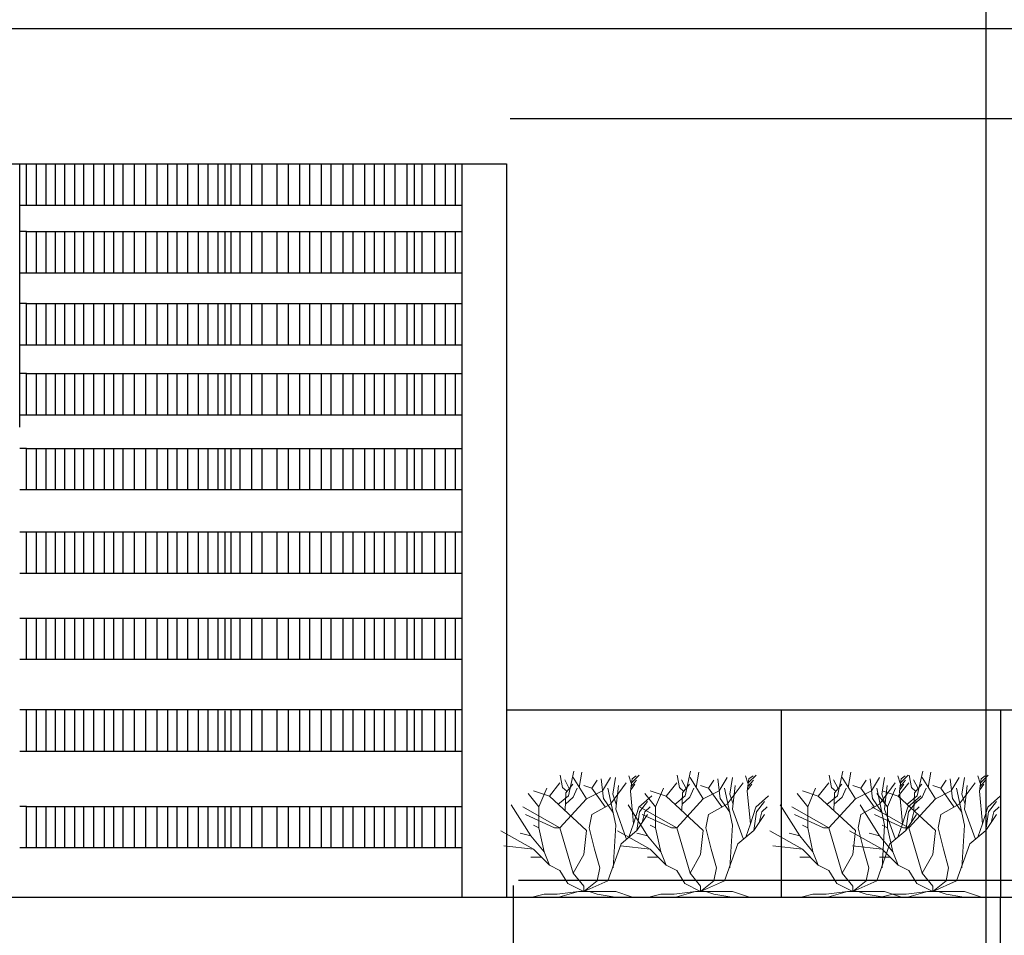
# Model space of a CAD drawing. Units: inches. Extents: x -117 to 121, y -77 to 40.
# Tile 34 of 45: x 45.7 to 57.65, y 10.29 to 21.42. Entities that reach past the tile are written whole.
import ezdxf

# ---------------------------------------------------------------- set-up
doc = ezdxf.new("R2010")
doc.units = ezdxf.units.IN
doc.header["$MEASUREMENT"] = 0
for name, color, linetype, lineweight in [('A-ANNO-DIMS', 2, 'Continuous', 18), ('A-ELEV', 7, 'Continuous', 25), ('L-PLNT', 3, 'Continuous', 13)]:
    doc.layers.add(name, color=color, linetype=linetype, lineweight=lineweight)
doc.styles.get("Standard").update_dxf_attribs({"font": 'arial.ttf'})
doc.dimstyles.get("Standard").update_dxf_attribs({"dimtxt": 0.18, "dimasz": 0.18, "dimexe": 0.18, "dimexo": 0.0625, "dimgap": 0.09, "dimtad": 0, "dimtih": 1, "dimtoh": 1, "dimdec": 4, "dimzin": 0, "dimdsep": 46, "dimtxsty": 'Standard', "dimcen": 0.09, "dimadec": 0, "dimazin": 0, "dimtfac": 1, "dimtdec": 4, "dimtofl": 0, "dimtmove": 0, "dimatfit": 3, "dimfxl": 1, "dimtolj": 1, "dimtzin": 0, "dimarcsym": 0})

# ---------------------------------------------------------------- blocks, each defined once
blk = doc.blocks.new('*U3')
for p, q in [((-12.471, 19.775), (-12.898, 22.044)), ((-11.433, 18.289), (-10.457, 22.749)), ((-8.16, 17.76), (-10.56, 21.6)), ((-9.48, 19.775), (-8.992, 22.592)), ((-5.28, 19.2), (-3.84, 21.6)), ((-3.377, 18.602), (-2.888, 21.575)), ((-0.508, 21.888), (-0.081, 20.558)), ((0.041, 20.714), (1.384, 22.044)), ((0.102, 21.34), (0.835, 21.888)), ((-16.8, 16.32), (-15.36, 19.68)), ((-14.88, 18.24), (-12.96, 20.64)), ((-11.677, 19.071), (-12.471, 19.775)), ((-11.28, 19.619), (-12.104, 21.184)), ((-11.921, 18.836), (-10.64, 20.401)), ((-10.579, 18.054), (-9.846, 19.697)), ((-7.2, 19.68), (-8.64, 20.16)), ((-7.2, 19.68), (-6.24, 21.12)), ((-4.8, 16.32), (-7.2, 19.68)), ((-5.086, 17.741), (-5.513, 21.34)), ((-2.88, 12.96), (-4.32, 19.68)), ((-3.84, 16.8), (-0.96, 20.64)), ((-2.88, 15.84), (-2.4, 20.16)), ((-0.203, 19.149), (0.102, 21.34)), ((-0.142, 19.384), (0.59, 20.401)), ((-0.02, 20.01), (0.896, 21.105)), ((-16.8, 16.32), (-18.72, 18.72)), ((-14.88, 18.24), (-17.76, 19.2)), ((-8.16, 12), (-14.88, 18.24)), ((-13.325, 16.724), (-11.433, 18.289)), ((-12.043, 15.628), (-11.921, 18.836)), ((-11.982, 16.802), (-10.579, 18.054)), ((-8.16, 17.76), (-5.28, 19.2)), ((-3.377, 15.315), (-5.086, 17.819)), ((-2.766, 16.802), (-3.377, 18.602)), ((0.346, 13.203), (-0.203, 19.149)), ((1.323, 16.254), (3.642, 18.289)), ((-18.24, 11.04), (-21.755, 16.655)), ((-12.96, 12.48), (-19.68, 16.32)), ((-16.8, 12.48), (-16.8, 16.32)), ((-12.96, 12.48), (-8.16, 17.76)), ((-7.2, 14.88), (-3.84, 16.8)), ((0.346, 13.203), (1.323, 16.254)), ((1.44, 15.36), (2.88, 17.28)), ((2.4, 15.36), (3.36, 16.32)), ((-13.92, 12.48), (-19.2, 14.88)), ((-7.68, 12.48), (-7.2, 14.88)), ((-0.96, 10.56), (-2.88, 15.84)), ((0.96, 12), (1.44, 15.36)), ((0.96, 12), (2.88, 14.88)), ((1.92, 13.44), (2.4, 15.36)), ((-16.8, 12.48), (-17.76, 12.96)), ((-15.84, 8.16), (-16.8, 12.48)), ((-12.96, 12.48), (-13.92, 12.48)), ((-10.56, 4.32), (-12.96, 12.48)), ((-6.72, 8.64), (-7.68, 12.48)), ((-3.36, 5.28), (-2.88, 12.96)), ((-0.48, 10.8), (0.346, 13.203)), ((-17.76, 8.64), (-23.663, 11.961)), ((-18.24, 11.04), (-20.16, 11.52)), ((-15.84, 8.16), (-18.24, 11.04)), ((-8.64, 7.68), (-8.16, 12)), ((-1.92, 9.6), (0.96, 12)), ((-17.76, 8.64), (-23.128, 9.222)), ((-4.32, 2.88), (-1.92, 9.6)), ((-16.32, 7.2), (-18.24, 7.2)), ((-14.88, 5.76), (-17.76, 8.64)), ((-14.88, 5.76), (-15.84, 8.16)), ((-10.56, 4.32), (-8.64, 7.68)), ((-5.76, 5.28), (-6.72, 8.64)), ((-12.96, 4.8), (-14.88, 5.76)), ((-11.52, 2.4), (-12.96, 4.8)), ((-8.64, 1.92), (-10.56, 4.32)), ((-6.24, 2.88), (-5.76, 5.28)), ((-8.64, 0.96), (-11.52, 2.4)), ((-8.64, 0.96), (-4.32, 2.88)), ((-8.64, 0.96), (-6.24, 2.88)), ((-8.64, 0.96), (-8.64, 1.92)), ((-15.84, 0.48), (-17.76, 0)), ((-13.44, 0.48), (-15.84, 0.48)), ((-9.6, 0.96), (-13.44, 0.48)), ((-9.6, 0.96), (-12.96, 0)), ((-9.6, 0.96), (-7.68, 0.96)), ((-8.64, 0.96), (-2.88, 0.96)), ((-7.68, 0.96), (-6.24, 0.48)), ((-6.24, 0.48), (-3.36, 0)), ((-2.88, 0.96), (0, 0))]:
    blk.add_line(p, q)
blk = doc.blocks.new('*D33')
at = {"layer": 'A-ANNO-DIMS', "color": 0, "lineweight": -2, "transparency": 16777216}
for p, q in [((57.433, -43.571), (57.433, 38.61)), ((70.621, -43.571), (70.621, 38.61)), ((57.613, 38.43), (63.572, 38.43)), ((70.441, 38.43), (64.482, 38.43))]:
    blk.add_line(p, q, dxfattribs=at)
at = {"layer": 'A-ANNO-DIMS', "color": 0, "transparency": 16777216}
for points in [[(57.613, 38.46), (57.613, 38.4), (57.433, 38.43)], [(70.441, 38.46), (70.441, 38.4), (70.621, 38.43)]]:
    blk.add_solid(points, dxfattribs=at)
at = {"layer": 'Defpoints', "color": 0, "transparency": 16777216}
for p in [(70.621, 38.43), (57.433, -43.633), (70.621, -43.633)]:
    blk.add_point(p, dxfattribs=at)
at = {"layer": 'A-ANNO-DIMS', "color": 0, "transparency": 16777216, "insert": (64.027, 38.43), "char_height": 0.18, "attachment_point": 5}
blk.add_mtext('\\A1;13.189', dxfattribs=at)
blk = doc.blocks.new('*D53')
at = {"layer": 'A-ANNO-DIMS', "color": 0, "lineweight": -2, "transparency": 16777216}
for p, q in [((51.69, 10.9), (51.69, -77.193)), ((27.974, 10.841), (27.974, -77.193)), ((28.154, -77.013), (39.367, -77.013)), ((51.51, -77.013), (40.297, -77.013))]:
    blk.add_line(p, q, dxfattribs=at)
at = {"layer": 'A-ANNO-DIMS', "color": 0, "transparency": 16777216}
for points in [[(28.154, -76.983), (28.154, -77.043), (27.974, -77.013)], [(51.51, -76.983), (51.51, -77.043), (51.69, -77.013)]]:
    blk.add_solid(points, dxfattribs=at)
at = {"layer": 'Defpoints', "color": 0, "transparency": 16777216}
for p in [(27.974, 10.903), (51.69, 10.962), (51.69, -77.013)]:
    blk.add_point(p, dxfattribs=at)
at = {"layer": 'A-ANNO-DIMS', "color": 0, "transparency": 16777216, "insert": (39.832, -77.013), "char_height": 0.18, "attachment_point": 5}
blk.add_mtext('\\A1;23.716', dxfattribs=at)
blk = doc.blocks.new('*D54')
at = {"layer": 'A-ANNO-DIMS', "color": 0, "lineweight": -2, "transparency": 16777216}
for p, q in [((51.654, 20.218), (120.84, 20.218)), ((120.66, 20.038), (120.66, 15.772)), ((120.66, 11.142), (120.66, 15.408)), ((51.753, 10.962), (120.84, 10.962))]:
    blk.add_line(p, q, dxfattribs=at)
at = {"layer": 'A-ANNO-DIMS', "color": 0, "transparency": 16777216}
for points in [[(120.63, 20.038), (120.69, 20.038), (120.66, 20.218)], [(120.63, 11.142), (120.69, 11.142), (120.66, 10.962)]]:
    blk.add_solid(points, dxfattribs=at)
at = {"layer": 'Defpoints', "color": 0, "transparency": 16777216}
for p in [(51.591, 20.218), (120.66, 20.218), (51.69, 10.962)]:
    blk.add_point(p, dxfattribs=at)
at = {"layer": 'A-ANNO-DIMS', "color": 0, "transparency": 16777216, "insert": (120.66, 15.59), "char_height": 0.18, "attachment_point": 5}
blk.add_mtext('\\A1;9.256', dxfattribs=at)

msp = doc.modelspace()

# ---------------------------------------------------------------- linework, layer by layer
at = {"layer": 'A-ELEV'}
for p, q in [((32.0351, 21.3104), (70.6115, 21.3104)), ((27.8529, 19.6653), (51.6089, 19.6653)), ((45.6984, 16.4655), (45.6984, 19.6653)), ((45.7795, 19.1644), (45.7795, 19.6653)), ((45.9016, 19.1644), (45.9016, 19.6653)), ((46.016, 19.1644), (46.016, 19.6653)), ((46.1303, 19.1644), (46.1303, 19.6653)), ((46.2447, 19.1644), (46.2447, 19.6653)), ((46.3668, 19.1644), (46.3668, 19.6653)), ((46.4735, 19.1644), (46.4735, 19.6653)), ((46.5955, 19.1644), (46.5955, 19.6653)), ((46.7252, 19.1644), (46.7252, 19.6653)), ((46.8396, 19.1644), (46.8396, 19.6653)), ((46.954, 19.1644), (46.954, 19.6653)), ((47.0912, 19.1644), (47.0912, 19.6653)), ((47.2285, 19.1644), (47.2285, 19.6653)), ((47.3658, 19.1644), (47.3658, 19.6653)), ((47.4954, 19.1644), (47.4954, 19.6653)), ((47.6098, 19.1644), (47.6098, 19.6653)), ((47.7395, 19.1644), (47.7395, 19.6653)), ((47.8691, 19.1644), (47.8691, 19.6653)), ((47.9835, 19.1644), (47.9835, 19.6653)), ((48.1055, 19.1644), (48.1055, 19.6653)), ((48.1933, 19.1644), (48.1933, 19.6562)), ((48.2657, 19.1644), (48.2657, 19.6653)), ((48.3724, 19.1644), (48.3724, 19.6653)), ((48.5173, 19.1644), (48.5173, 19.6653)), ((48.6394, 19.1644), (48.6394, 19.6653)), ((48.8224, 19.1644), (48.8224, 19.6653)), ((48.9597, 19.1644), (48.9597, 19.6653)), ((49.0969, 19.1644), (49.0969, 19.6653)), ((49.219, 19.1644), (49.219, 19.6653)), ((49.3638, 19.1644), (49.3638, 19.6653)), ((49.4782, 19.1644), (49.4782, 19.6653)), ((49.6231, 19.1644), (49.6231, 19.6653)), ((49.7452, 19.1644), (49.7452, 19.6653)), ((49.8901, 19.1644), (49.8901, 19.6653)), ((50.0044, 19.1644), (50.0044, 19.6653)), ((50.1265, 19.1644), (50.1265, 19.6653)), ((50.2561, 19.1644), (50.2561, 19.6653)), ((50.401, 19.1644), (50.401, 19.6653)), ((50.4925, 19.1644), (50.4925, 19.6653)), ((50.584, 19.1644), (50.584, 19.6653)), ((50.7366, 19.1644), (50.7366, 19.6653)), ((50.8662, 19.1644), (50.8662, 19.6653)), ((50.9882, 19.1644), (50.9882, 19.6653)), ((51.0706, 10.755), (51.0706, 19.6653)), ((51.6089, 19.6653), (51.6089, 10.755)), ((45.6984, 19.1644), (51.0706, 19.1644)), ((45.7795, 18.8424), (45.6984, 18.8424)), ((45.7795, 18.3415), (45.7795, 18.8424)), ((45.7795, 18.8424), (51.0706, 18.8424)), ((45.9016, 18.3415), (45.9016, 18.8424)), ((46.016, 18.3415), (46.016, 18.8424)), ((46.1303, 18.3415), (46.1303, 18.8424)), ((46.2447, 18.3415), (46.2447, 18.8424)), ((46.3668, 18.3415), (46.3668, 18.8424)), ((46.4735, 18.3415), (46.4735, 18.8424)), ((46.5955, 18.3415), (46.5955, 18.8424)), ((46.7252, 18.3415), (46.7252, 18.8424)), ((46.8396, 18.3415), (46.8396, 18.8424)), ((46.954, 18.3415), (46.954, 18.8424)), ((47.0912, 18.3415), (47.0912, 18.8424)), ((47.2285, 18.3415), (47.2285, 18.8424)), ((47.3658, 18.3415), (47.3658, 18.8424)), ((47.4954, 18.3415), (47.4954, 18.8424)), ((47.6098, 18.3415), (47.6098, 18.8424)), ((47.7395, 18.3415), (47.7395, 18.8424)), ((47.8691, 18.3415), (47.8691, 18.8424)), ((47.9835, 18.3415), (47.9835, 18.8424)), ((48.1055, 18.3415), (48.1055, 18.8424)), ((48.1933, 18.3415), (48.1933, 18.8333)), ((48.2657, 18.3415), (48.2657, 18.8424)), ((48.3724, 18.3415), (48.3724, 18.8424)), ((48.5173, 18.3415), (48.5173, 18.8424)), ((48.6394, 18.3415), (48.6394, 18.8424)), ((48.8224, 18.3415), (48.8224, 18.8424)), ((48.9597, 18.3415), (48.9597, 18.8424)), ((49.0969, 18.3415), (49.0969, 18.8424)), ((49.219, 18.3415), (49.219, 18.8424)), ((49.3638, 18.3415), (49.3638, 18.8424)), ((49.4782, 18.3415), (49.4782, 18.8424)), ((49.6231, 18.3415), (49.6231, 18.8424)), ((49.7452, 18.3415), (49.7452, 18.8424)), ((49.8901, 18.3415), (49.8901, 18.8424)), ((50.0044, 18.3415), (50.0044, 18.8424)), ((50.1265, 18.3415), (50.1265, 18.8424)), ((50.2561, 18.3415), (50.2561, 18.8424)), ((50.401, 18.3415), (50.401, 18.8424)), ((50.4925, 18.3415), (50.4925, 18.8424)), ((50.584, 18.3415), (50.584, 18.8424)), ((50.7366, 18.3415), (50.7366, 18.8424)), ((50.8662, 18.3415), (50.8662, 18.8424)), ((50.9882, 18.3415), (50.9882, 18.8424)), ((45.6984, 18.3415), (51.0706, 18.3415)), ((45.7795, 17.9696), (45.6984, 17.9696)), ((45.7795, 17.4687), (45.7795, 17.9696)), ((45.7795, 17.9696), (51.0706, 17.9696)), ((45.9016, 17.4687), (45.9016, 17.9696)), ((46.016, 17.4687), (46.016, 17.9696)), ((46.1303, 17.4687), (46.1303, 17.9696)), ((46.2447, 17.4687), (46.2447, 17.9696)), ((46.3668, 17.4687), (46.3668, 17.9696)), ((46.4735, 17.4687), (46.4735, 17.9696)), ((46.5955, 17.4687), (46.5955, 17.9696)), ((46.7252, 17.4687), (46.7252, 17.9696)), ((46.8396, 17.4687), (46.8396, 17.9696)), ((46.954, 17.4687), (46.954, 17.9696)), ((47.0912, 17.4687), (47.0912, 17.9696)), ((47.2285, 17.4687), (47.2285, 17.9696)), ((47.3658, 17.4687), (47.3658, 17.9696)), ((47.4954, 17.4687), (47.4954, 17.9696)), ((47.6098, 17.4687), (47.6098, 17.9696)), ((47.7395, 17.4687), (47.7395, 17.9696)), ((47.8691, 17.4687), (47.8691, 17.9696)), ((47.9835, 17.4687), (47.9835, 17.9696)), ((48.1055, 17.4687), (48.1055, 17.9696)), ((48.1933, 17.4687), (48.1933, 17.9605)), ((48.2657, 17.4687), (48.2657, 17.9696)), ((48.3724, 17.4687), (48.3724, 17.9696)), ((48.5173, 17.4687), (48.5173, 17.9696)), ((48.6394, 17.4687), (48.6394, 17.9696)), ((48.8224, 17.4687), (48.8224, 17.9696)), ((48.9597, 17.4687), (48.9597, 17.9696)), ((49.0969, 17.4687), (49.0969, 17.9696)), ((49.219, 17.4687), (49.219, 17.9696)), ((49.3638, 17.4687), (49.3638, 17.9696)), ((49.4782, 17.4687), (49.4782, 17.9696)), ((49.6231, 17.4687), (49.6231, 17.9696)), ((49.7452, 17.4687), (49.7452, 17.9696)), ((49.8901, 17.4687), (49.8901, 17.9696)), ((50.0044, 17.4687), (50.0044, 17.9696)), ((50.1265, 17.4687), (50.1265, 17.9696)), ((50.2561, 17.4687), (50.2561, 17.9696)), ((50.401, 17.4687), (50.401, 17.9696)), ((50.4925, 17.4687), (50.4925, 17.9696)), ((50.584, 17.4687), (50.584, 17.9696)), ((50.7366, 17.4687), (50.7366, 17.9696)), ((50.8662, 17.4687), (50.8662, 17.9696)), ((50.9882, 17.4687), (50.9882, 17.9696)), ((45.6984, 17.4687), (51.0706, 17.4687)), ((45.7795, 17.1187), (45.6984, 17.1187)), ((45.7795, 16.6179), (45.7795, 17.1187)), ((45.7795, 17.1187), (51.0706, 17.1187)), ((45.9016, 16.6179), (45.9016, 17.1187)), ((46.016, 16.6179), (46.016, 17.1187)), ((46.1303, 16.6179), (46.1303, 17.1187)), ((46.2447, 16.6179), (46.2447, 17.1187)), ((46.3668, 16.6179), (46.3668, 17.1187)), ((46.4735, 16.6179), (46.4735, 17.1187)), ((46.5955, 16.6179), (46.5955, 17.1187)), ((46.7252, 16.6179), (46.7252, 17.1187)), ((46.8396, 16.6179), (46.8396, 17.1187)), ((46.954, 16.6179), (46.954, 17.1187)), ((47.0912, 16.6179), (47.0912, 17.1187)), ((47.2285, 16.6179), (47.2285, 17.1187)), ((47.3658, 16.6179), (47.3658, 17.1187)), ((47.4954, 16.6179), (47.4954, 17.1187)), ((47.6098, 16.6179), (47.6098, 17.1187)), ((47.7395, 16.6179), (47.7395, 17.1187)), ((47.8691, 16.6179), (47.8691, 17.1187)), ((47.9835, 16.6179), (47.9835, 17.1187)), ((48.1055, 16.6179), (48.1055, 17.1187)), ((48.1933, 16.6179), (48.1933, 17.1097)), ((48.2657, 16.6179), (48.2657, 17.1187)), ((48.3724, 16.6179), (48.3724, 17.1187)), ((48.5173, 16.6179), (48.5173, 17.1187)), ((48.6394, 16.6179), (48.6394, 17.1187)), ((48.8224, 16.6179), (48.8224, 17.1187)), ((48.9597, 16.6179), (48.9597, 17.1187)), ((49.0969, 16.6179), (49.0969, 17.1187)), ((49.219, 16.6179), (49.219, 17.1187)), ((49.3638, 16.6179), (49.3638, 17.1187)), ((49.4782, 16.6179), (49.4782, 17.1187)), ((49.6231, 16.6179), (49.6231, 17.1187)), ((49.7452, 16.6179), (49.7452, 17.1187)), ((49.8901, 16.6179), (49.8901, 17.1187)), ((50.0044, 16.6179), (50.0044, 17.1187)), ((50.1265, 16.6179), (50.1265, 17.1187)), ((50.2561, 16.6179), (50.2561, 17.1187)), ((50.401, 16.6179), (50.401, 17.1187)), ((50.4925, 16.6179), (50.4925, 17.1187)), ((50.584, 16.6179), (50.584, 17.1187)), ((50.7366, 16.6179), (50.7366, 17.1187)), ((50.8662, 16.6179), (50.8662, 17.1187)), ((50.9882, 16.6179), (50.9882, 17.1187)), ((45.6984, 16.6179), (51.0706, 16.6179)), ((45.7795, 16.2085), (45.6984, 16.2085)), ((45.7795, 15.7077), (45.7795, 16.2085)), ((45.7795, 16.2085), (51.0706, 16.2085)), ((45.9016, 15.7077), (45.9016, 16.2085)), ((46.016, 15.7077), (46.016, 16.2085)), ((46.1303, 15.7077), (46.1303, 16.2085)), ((46.2447, 15.7077), (46.2447, 16.2085)), ((46.3668, 15.7077), (46.3668, 16.2085)), ((46.4735, 15.7077), (46.4735, 16.2085)), ((46.5955, 15.7077), (46.5955, 16.2085)), ((46.7252, 15.7077), (46.7252, 16.2085)), ((46.8396, 15.7077), (46.8396, 16.2085)), ((46.954, 15.7077), (46.954, 16.2085)), ((47.0912, 15.7077), (47.0912, 16.2085)), ((47.2285, 15.7077), (47.2285, 16.2085)), ((47.3658, 15.7077), (47.3658, 16.2085)), ((47.4954, 15.7077), (47.4954, 16.2085)), ((47.6098, 15.7077), (47.6098, 16.2085)), ((47.7395, 15.7077), (47.7395, 16.2085)), ((47.8691, 15.7077), (47.8691, 16.2085)), ((47.9835, 15.7077), (47.9835, 16.2085)), ((48.1055, 15.7077), (48.1055, 16.2085)), ((48.1933, 15.7077), (48.1933, 16.1995)), ((48.2657, 15.7077), (48.2657, 16.2085)), ((48.3724, 15.7077), (48.3724, 16.2085)), ((48.5173, 15.7077), (48.5173, 16.2085)), ((48.6394, 15.7077), (48.6394, 16.2085)), ((48.8224, 15.7077), (48.8224, 16.2085)), ((48.9597, 15.7077), (48.9597, 16.2085)), ((49.0969, 15.7077), (49.0969, 16.2085)), ((49.219, 15.7077), (49.219, 16.2085)), ((49.3638, 15.7077), (49.3638, 16.2085)), ((49.4782, 15.7077), (49.4782, 16.2085)), ((49.6231, 15.7077), (49.6231, 16.2085)), ((49.7452, 15.7077), (49.7452, 16.2085)), ((49.8901, 15.7077), (49.8901, 16.2085)), ((50.0044, 15.7077), (50.0044, 16.2085)), ((50.1265, 15.7077), (50.1265, 16.2085)), ((50.2561, 15.7077), (50.2561, 16.2085)), ((50.401, 15.7077), (50.401, 16.2085)), ((50.4925, 15.7077), (50.4925, 16.2085)), ((50.584, 15.7077), (50.584, 16.2085)), ((50.7366, 15.7077), (50.7366, 16.2085)), ((50.8662, 15.7077), (50.8662, 16.2085)), ((50.9882, 15.7077), (50.9882, 16.2085)), ((45.6984, 15.7077), (51.0706, 15.7077)), ((45.6984, 15.1944), (51.0706, 15.1944)), ((45.7795, 14.6936), (45.7795, 15.1944)), ((45.9016, 14.6936), (45.9016, 15.1944)), ((46.016, 14.6936), (46.016, 15.1944)), ((46.1303, 14.6936), (46.1303, 15.1944)), ((46.2447, 14.6936), (46.2447, 15.1944)), ((46.3668, 14.6936), (46.3668, 15.1944)), ((46.4735, 14.6936), (46.4735, 15.1944)), ((46.5955, 14.6936), (46.5955, 15.1944)), ((46.7252, 14.6936), (46.7252, 15.1944)), ((46.8396, 14.6936), (46.8396, 15.1944)), ((46.954, 14.6936), (46.954, 15.1944)), ((47.0912, 14.6936), (47.0912, 15.1944)), ((47.2285, 14.6936), (47.2285, 15.1944)), ((47.3658, 14.6936), (47.3658, 15.1944)), ((47.4954, 14.6936), (47.4954, 15.1944)), ((47.6098, 14.6936), (47.6098, 15.1944)), ((47.7395, 14.6936), (47.7395, 15.1944)), ((47.8691, 14.6936), (47.8691, 15.1944)), ((47.9835, 14.6936), (47.9835, 15.1944)), ((48.1055, 14.6936), (48.1055, 15.1944)), ((48.2657, 14.6936), (48.2657, 15.1944)), ((48.3724, 14.6936), (48.3724, 15.1944)), ((48.5173, 14.6936), (48.5173, 15.1944)), ((48.6394, 14.6936), (48.6394, 15.1944)), ((48.8224, 14.6936), (48.8224, 15.1944)), ((48.9597, 14.6936), (48.9597, 15.1944)), ((49.0969, 14.6936), (49.0969, 15.1944)), ((49.219, 14.6936), (49.219, 15.1944)), ((49.3638, 14.6936), (49.3638, 15.1944)), ((49.4782, 14.6936), (49.4782, 15.1944)), ((49.6231, 14.6936), (49.6231, 15.1944)), ((49.7452, 14.6936), (49.7452, 15.1944)), ((49.8901, 14.6936), (49.8901, 15.1944)), ((50.0044, 14.6936), (50.0044, 15.1944)), ((50.1265, 14.6936), (50.1265, 15.1944)), ((50.2561, 14.6936), (50.2561, 15.1944)), ((50.401, 14.6936), (50.401, 15.1944)), ((50.4925, 14.6936), (50.4925, 15.1944)), ((50.584, 14.6936), (50.584, 15.1944)), ((50.7366, 14.6936), (50.7366, 15.1944)), ((50.8662, 14.6936), (50.8662, 15.1944)), ((50.9882, 14.6936), (50.9882, 15.1944)), ((48.1933, 14.6936), (48.1933, 15.1854)), ((45.6984, 14.6936), (51.0706, 14.6936)), ((45.6984, 14.1471), (51.0706, 14.1471)), ((45.7795, 13.6462), (45.7795, 14.1471)), ((45.9016, 13.6462), (45.9016, 14.1471)), ((46.016, 13.6462), (46.016, 14.1471)), ((46.1303, 13.6462), (46.1303, 14.1471)), ((46.2447, 13.6462), (46.2447, 14.1471)), ((46.3668, 13.6462), (46.3668, 14.1471)), ((46.4735, 13.6462), (46.4735, 14.1471)), ((46.5955, 13.6462), (46.5955, 14.1471)), ((46.7252, 13.6462), (46.7252, 14.1471)), ((46.8396, 13.6462), (46.8396, 14.1471)), ((46.954, 13.6462), (46.954, 14.1471)), ((47.0912, 13.6462), (47.0912, 14.1471)), ((47.2285, 13.6462), (47.2285, 14.1471)), ((47.3658, 13.6462), (47.3658, 14.1471)), ((47.4954, 13.6462), (47.4954, 14.1471)), ((47.6098, 13.6462), (47.6098, 14.1471)), ((47.7395, 13.6462), (47.7395, 14.1471)), ((47.8691, 13.6462), (47.8691, 14.1471)), ((47.9835, 13.6462), (47.9835, 14.1471)), ((48.1055, 13.6462), (48.1055, 14.1471)), ((48.1933, 13.6462), (48.1933, 14.138)), ((48.2657, 13.6462), (48.2657, 14.1471)), ((48.3724, 13.6462), (48.3724, 14.1471)), ((48.5173, 13.6462), (48.5173, 14.1471)), ((48.6394, 13.6462), (48.6394, 14.1471)), ((48.8224, 13.6462), (48.8224, 14.1471)), ((48.9597, 13.6462), (48.9597, 14.1471)), ((49.0969, 13.6462), (49.0969, 14.1471)), ((49.219, 13.6462), (49.219, 14.1471)), ((49.3638, 13.6462), (49.3638, 14.1471)), ((49.4782, 13.6462), (49.4782, 14.1471)), ((49.6231, 13.6462), (49.6231, 14.1471)), ((49.7452, 13.6462), (49.7452, 14.1471)), ((49.8901, 13.6462), (49.8901, 14.1471)), ((50.0044, 13.6462), (50.0044, 14.1471)), ((50.1265, 13.6462), (50.1265, 14.1471)), ((50.2561, 13.6462), (50.2561, 14.1471)), ((50.401, 13.6462), (50.401, 14.1471)), ((50.4925, 13.6462), (50.4925, 14.1471)), ((50.584, 13.6462), (50.584, 14.1471)), ((50.7366, 13.6462), (50.7366, 14.1471)), ((50.8662, 13.6462), (50.8662, 14.1471)), ((50.9882, 13.6462), (50.9882, 14.1471)), ((45.6984, 13.6462), (51.0706, 13.6462)), ((51.0706, 13.0312), (45.6984, 13.0312)), ((45.7795, 12.5304), (45.7795, 13.0312)), ((45.9016, 12.5304), (45.9016, 13.0312)), ((46.016, 12.5304), (46.016, 13.0312)), ((46.1303, 12.5304), (46.1303, 13.0312)), ((46.2447, 12.5304), (46.2447, 13.0312)), ((46.3668, 12.5304), (46.3668, 13.0312)), ((46.4735, 12.5304), (46.4735, 13.0312)), ((46.5955, 12.5304), (46.5955, 13.0312)), ((46.7252, 12.5304), (46.7252, 13.0312)), ((46.8396, 12.5304), (46.8396, 13.0312)), ((46.954, 12.5304), (46.954, 13.0312)), ((47.0912, 12.5304), (47.0912, 13.0312)), ((47.2285, 12.5304), (47.2285, 13.0312)), ((47.3658, 12.5304), (47.3658, 13.0312)), ((47.4954, 12.5304), (47.4954, 13.0312)), ((47.6098, 12.5304), (47.6098, 13.0312)), ((47.7395, 12.5304), (47.7395, 13.0312)), ((47.8691, 12.5304), (47.8691, 13.0312)), ((47.9835, 12.5304), (47.9835, 13.0312)), ((48.1055, 12.5304), (48.1055, 13.0312)), ((48.1933, 12.5304), (48.1933, 13.0221)), ((48.2657, 12.5304), (48.2657, 13.0312)), ((48.3724, 12.5304), (48.3724, 13.0312)), ((48.5173, 12.5304), (48.5173, 13.0312)), ((48.6394, 12.5304), (48.6394, 13.0312)), ((48.8224, 12.5304), (48.8224, 13.0312)), ((48.9597, 12.5304), (48.9597, 13.0312)), ((49.0969, 12.5304), (49.0969, 13.0312)), ((49.219, 12.5304), (49.219, 13.0312)), ((49.3638, 12.5304), (49.3638, 13.0312)), ((49.4782, 12.5304), (49.4782, 13.0312)), ((49.6231, 12.5304), (49.6231, 13.0312)), ((49.7452, 12.5304), (49.7452, 13.0312)), ((49.8901, 12.5304), (49.8901, 13.0312)), ((50.0044, 12.5304), (50.0044, 13.0312)), ((50.1265, 12.5304), (50.1265, 13.0312)), ((50.2561, 12.5304), (50.2561, 13.0312)), ((50.401, 12.5304), (50.401, 13.0312)), ((50.4925, 12.5304), (50.4925, 13.0312)), ((50.584, 12.5304), (50.584, 13.0312)), ((50.7366, 12.5304), (50.7366, 13.0312)), ((50.8662, 12.5304), (50.8662, 13.0312)), ((50.9882, 12.5304), (50.9882, 13.0312)), ((51.6089, 13.0312), (81.0386, 13.0312)), ((54.943, 13.0312), (54.943, 10.755)), ((57.6104, 13.0312), (57.6104, 10.755)), ((45.6984, 12.5304), (51.0706, 12.5304)), ((45.7795, 11.8591), (45.6984, 11.8591)), ((45.7795, 11.3583), (45.7795, 11.8591)), ((45.7795, 11.8591), (51.0706, 11.8591)), ((45.9016, 11.3583), (45.9016, 11.8591)), ((46.016, 11.3583), (46.016, 11.8591)), ((46.1303, 11.3583), (46.1303, 11.8591)), ((46.2447, 11.3583), (46.2447, 11.8591)), ((46.3668, 11.3583), (46.3668, 11.8591)), ((46.4735, 11.3583), (46.4735, 11.8591)), ((46.5955, 11.3583), (46.5955, 11.8591)), ((46.7252, 11.3583), (46.7252, 11.8591)), ((46.8396, 11.3583), (46.8396, 11.8591)), ((46.954, 11.3583), (46.954, 11.8591)), ((47.0912, 11.3583), (47.0912, 11.8591)), ((47.2285, 11.3583), (47.2285, 11.8591)), ((47.3658, 11.3583), (47.3658, 11.8591)), ((47.4954, 11.3583), (47.4954, 11.8591)), ((47.6098, 11.3583), (47.6098, 11.8591)), ((47.7395, 11.3583), (47.7395, 11.8591)), ((47.8691, 11.3583), (47.8691, 11.8591)), ((47.9835, 11.3583), (47.9835, 11.8591)), ((48.1055, 11.3583), (48.1055, 11.8591)), ((48.1933, 11.3583), (48.1933, 11.8501)), ((48.2657, 11.3583), (48.2657, 11.8591)), ((48.3724, 11.3583), (48.3724, 11.8591)), ((48.5173, 11.3583), (48.5173, 11.8591)), ((48.6394, 11.3583), (48.6394, 11.8591)), ((48.8224, 11.3583), (48.8224, 11.8591)), ((48.9597, 11.3583), (48.9597, 11.8591)), ((49.0969, 11.3583), (49.0969, 11.8591)), ((49.219, 11.3583), (49.219, 11.8591)), ((49.3638, 11.3583), (49.3638, 11.8591)), ((49.4782, 11.3583), (49.4782, 11.8591)), ((49.6231, 11.3583), (49.6231, 11.8591)), ((49.7452, 11.3583), (49.7452, 11.8591)), ((49.8901, 11.3583), (49.8901, 11.8591)), ((50.0044, 11.3583), (50.0044, 11.8591)), ((50.1265, 11.3583), (50.1265, 11.8591)), ((50.2561, 11.3583), (50.2561, 11.8591)), ((50.401, 11.3583), (50.401, 11.8591)), ((50.4925, 11.3583), (50.4925, 11.8591)), ((50.584, 11.3583), (50.584, 11.8591)), ((50.7366, 11.3583), (50.7366, 11.8591)), ((50.8662, 11.3583), (50.8662, 11.8591)), ((50.9882, 11.3583), (50.9882, 11.8591)), ((45.6984, 11.3583), (51.0706, 11.3583)), ((16.862, 10.755), (51.6089, 10.755)), ((51.6089, 10.755), (72.955, 10.755)), ((57.6104, 9.9998), (57.6104, 10.755))]:
    msp.add_line(p, q, dxfattribs=at)

# ---------------------------------------------------------------- block references
at = {"layer": 'L-PLNT', "xscale": 0.0671647796176818, "yscale": 0.0671647796176818, "zscale": 0.0671647796176818}
for p in [(53.1285, 10.7596), (54.5471, 10.7596), (56.3951, 10.7596), (57.3658, 10.7596)]:
    msp.add_blockref('*U3', p, dxfattribs=at)

# ---------------------------------------------------------------- dimensions: what is measured, and where the dimension line sits
at = {"layer": 'A-ANNO-DIMS'}
for base, p1, p2, picture, middle in [((70.6214, 38.4297), (57.4328, -43.6334), (70.6214, -43.6334), '*D33', (64.0271, 38.4297)), ((51.6901, -77.0135), (27.9744, 10.9032), (51.6901, 10.9623), '*D53', (39.8322, -77.0135))]:
    dim = msp.add_linear_dim(base=base, p1=p1, p2=p2, dimstyle='Standard', override={"dimdec": 3, "dimlfac": 1, "dimrnd": 0, "dimzin": 0, "dimdsep": 46, "dimlunit": 2}, dxfattribs=at)
    dim.commit()
    dim.dimension.update_dxf_attribs({"geometry": picture, "text_midpoint": middle})
dim = msp.add_linear_dim(base=(120.6602, 20.2181), p1=(51.6901, 10.9623), p2=(51.5915, 20.2181), angle=90, dimstyle='Standard', override={"dimdec": 3, "dimlfac": 1, "dimrnd": 0, "dimzin": 0, "dimdsep": 46, "dimlunit": 2}, dxfattribs=at)
dim.commit()
dim.dimension.update_dxf_attribs({"geometry": '*D54', "text_midpoint": (120.6602, 15.5902)})

doc.saveas('drawing.dxf')
